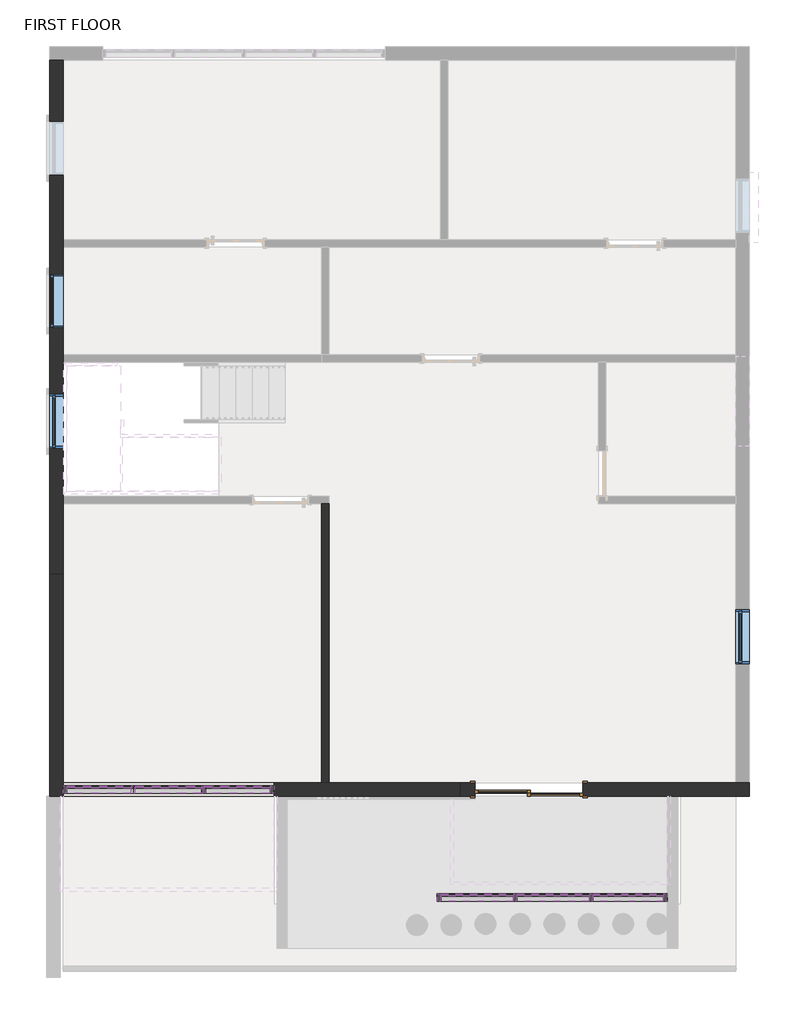
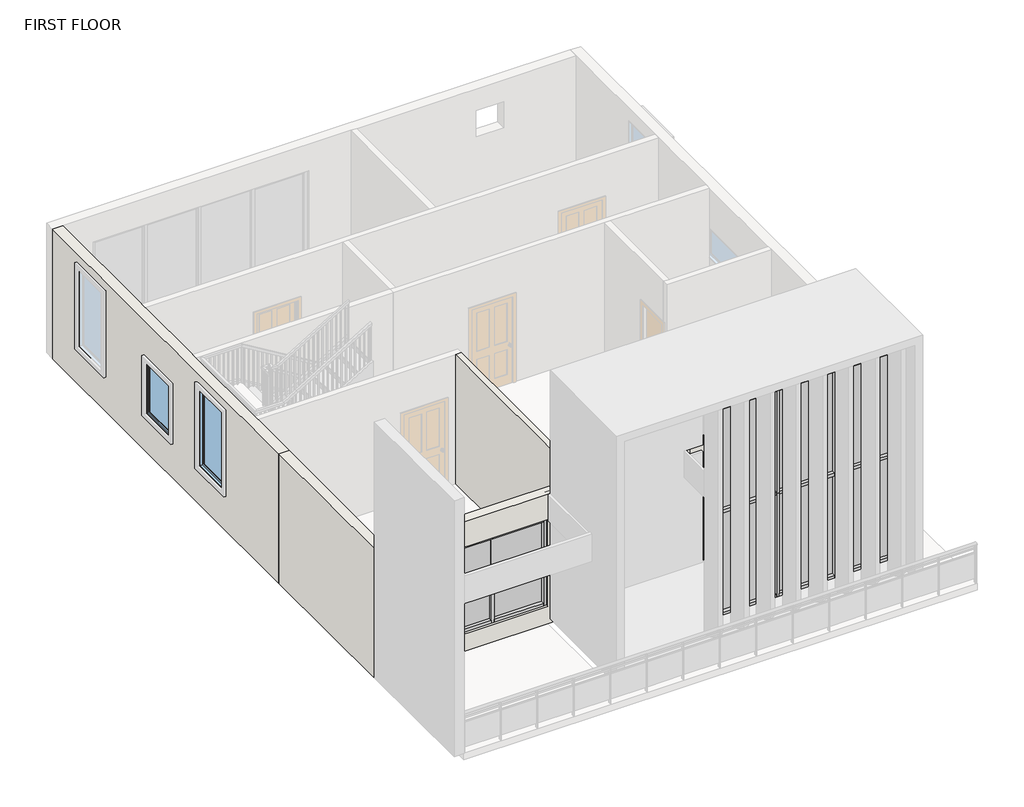
# One storey, part 1 of 4: 42 members, 15 plates, 6 walls, 3 windows, 1 door.
"""IFC4 building model written with IfcOpenShell, lengths in millimetres."""

from ifc_helpers import new_model, si_unit, frame, origin, place, context, project, spatial, polyline, outline, extrude, faceted_brep, transform, mapped, element, save
from components import door_d4d75d1e, member_f0fea5a5, member_ee409385, member_9476229c, member_234fa6b3, member_c6549b41, member_65ceef43, member_37269937, member_65519335, member_c344cd1a, member_3285b992, member_9e1336f4, member_2c52e315, member_a24dc69d, member_2a256751, member_8c482a5e, member_f4ce465c, member_cd6cc0cf, system_panel_glazed_74eece19, system_panel_glazed_8fc2b39e, system_panel_glazed_e38def25, system_panel_glazed_5eb7606f, system_panel_glazed_a48af828, system_panel_glazed_d044bda1, system_panel_glazed_a4577834, system_panel_glazed_3aabc813, system_panel_glazed_a3f6c58c, system_panel_glazed_533eadb3, system_panel_glazed_eb972c8e, system_panel_glazed_22820276, window_c1f32544, window_2e8ca8a3

model = new_model("IFC4")

# Units and contexts
model_context = context("Model", 3, world=origin())
ifc_project = project(units=[si_unit("LENGTHUNIT", "METRE", prefix="MILLI")], contexts=[model_context])

# Site, building, storey
site = spatial("IfcSite", under=ifc_project)
building = spatial("IfcBuilding", under=site)
storey = spatial("IfcBuildingStorey", under=building, Name="FIRST FLOOR", Elevation=3352.8)

# Door
placement = place(None, origin())
door_shape = door_d4d75d1e(model_context)
element("IfcDoor", 1, ObjectType="Door-Double-Sliding : 72\" x 84\"", at=placement, inside=storey, context=model_context, shape_type="MappedRepresentation", body=[
    mapped(door_shape, transform((-1851.8781265, -4147.9142532, 3352.8), x_axis=(-1.0, 0.0, 0.0), y_axis=(0.0, -1.0, 0.0), z_axis=(0.0, 0.0, 1.0))),
])

# Members
member_shape = member_f0fea5a5(model_context)
element("IfcMember", 2, ObjectType="Rectangular Mullion : 2.5\" x 5\" rectangular", at=placement, inside=storey, context=model_context, shape_type="MappedRepresentation", body=[
    mapped(member_shape, transform((-3373.3381264, -6103.7142532, 3631.9550828), x_axis=(1.0, 0.0, 0.0), y_axis=(0.0, -1.0, 0.0), z_axis=(0.0, 0.0, -1.0))),
])
element("IfcMember", 3, ObjectType="Rectangular Mullion : 2.5\" x 5\" rectangular", at=placement, inside=storey, context=model_context, shape_type="MappedRepresentation", body=[
    mapped(member_shape, transform((-2083.0181265, -6103.7142532, 3631.9550828), x_axis=(1.0, 0.0, 0.0), y_axis=(0.0, -1.0, 0.0), z_axis=(0.0, 0.0, -1.0))),
])
element("IfcMember", 4, ObjectType="Rectangular Mullion : 2.5\" x 5\" rectangular", at=placement, inside=storey, context=model_context, shape_type="MappedRepresentation", body=[
    mapped(member_shape, transform((-792.6981266, -6103.7142532, 3631.9550828), x_axis=(1.0, 0.0, 0.0), y_axis=(0.0, -1.0, 0.0), z_axis=(0.0, 0.0, -1.0))),
])
element("IfcMember", 5, ObjectType="Rectangular Mullion : 2.5\" x 5\" rectangular", at=placement, inside=storey, context=model_context, shape_type="MappedRepresentation", body=[
    mapped(member_shape, transform((-3373.3381264, -6103.7142532, 6070.3550828), x_axis=(1.0, 0.0, 0.0), y_axis=(0.0, -1.0, 0.0), z_axis=(0.0, 0.0, -1.0))),
])
element("IfcMember", 6, ObjectType="Rectangular Mullion : 2.5\" x 5\" rectangular", at=placement, inside=storey, context=model_context, shape_type="MappedRepresentation", body=[
    mapped(member_shape, transform((-2083.0181265, -6103.7142532, 6070.3550828), x_axis=(1.0, 0.0, 0.0), y_axis=(0.0, -1.0, 0.0), z_axis=(0.0, 0.0, -1.0))),
])
element("IfcMember", 7, ObjectType="Rectangular Mullion : 2.5\" x 5\" rectangular", at=placement, inside=storey, context=model_context, shape_type="MappedRepresentation", body=[
    mapped(member_shape, transform((-792.6981266, -6103.7142532, 6070.3550828), x_axis=(1.0, 0.0, 0.0), y_axis=(0.0, -1.0, 0.0), z_axis=(0.0, 0.0, -1.0))),
])
member_2_shape = member_ee409385(model_context)
element("IfcMember", 8, ObjectType="Rectangular Mullion : 2.5\" x 5\" rectangular", at=placement, inside=storey, context=model_context, shape_type="MappedRepresentation", body=[
    mapped(member_2_shape, transform((497.6218735, -6103.7142532, 3631.9550828), x_axis=(1.0, 0.0, 0.0), y_axis=(0.0, -1.0, 0.0), z_axis=(0.0, 0.0, -1.0))),
])
element("IfcMember", 9, ObjectType="Rectangular Mullion : 2.5\" x 5\" rectangular", at=placement, inside=storey, context=model_context, shape_type="MappedRepresentation", body=[
    mapped(member_2_shape, transform((497.6218735, -6103.7142532, 6070.3550828), x_axis=(1.0, 0.0, 0.0), y_axis=(0.0, -1.0, 0.0), z_axis=(0.0, 0.0, -1.0))),
])
element("IfcMember", 10, ObjectType="Rectangular Mullion : 2.5\" x 5\" rectangular", at=placement, inside=storey, context=model_context, shape_type="MappedRepresentation", body=[
    mapped(member_2_shape, transform((-3413.9781265, -6103.7142532, 6070.3550828), x_axis=(-1.0, 0.0, 0.0), y_axis=(0.0, -1.0, 0.0), z_axis=(0.0, 0.0, 1.0))),
])
element("IfcMember", 11, ObjectType="Rectangular Mullion : 2.5\" x 5\" rectangular", at=placement, inside=storey, context=model_context, shape_type="MappedRepresentation", body=[
    mapped(member_2_shape, transform((-3413.9781265, -6103.7142532, 8508.7550828), x_axis=(-1.0, 0.0, 0.0), y_axis=(0.0, -1.0, 0.0), z_axis=(0.0, 0.0, 1.0))),
])
member_3_shape = member_9476229c(model_context)
element("IfcMember", 12, ObjectType="Rectangular Mullion : 2.5\" x 5\" rectangular", at=placement, inside=storey, context=model_context, shape_type="MappedRepresentation", body=[
    mapped(member_3_shape, transform((434.1218735, -6103.7142532, 9132.458551), x_axis=(0.0, 0.0, 1.0), y_axis=(0.0, -1.0, 0.0), z_axis=(1.0, 0.0, 0.0))),
])
element("IfcMember", 13, ObjectType="Rectangular Mullion : 2.5\" x 5\" rectangular", at=placement, inside=storey, context=model_context, shape_type="MappedRepresentation", body=[
    mapped(member_3_shape, transform((-760.9481266, -6103.7142532, 3631.9550828), x_axis=(0.0, 0.0, -1.0), y_axis=(0.0, -1.0, 0.0), z_axis=(-1.0, 0.0, 0.0))),
])
member_4_shape = member_234fa6b3(model_context)
element("IfcMember", 14, ObjectType="Rectangular Mullion : 2.5\" x 5\" rectangular", at=placement, inside=storey, context=model_context, shape_type="MappedRepresentation", body=[
    mapped(member_4_shape, transform((-2114.7681265, -6103.7142532, 9132.458551), x_axis=(0.0, 0.0, 1.0), y_axis=(0.0, -1.0, 0.0), z_axis=(1.0, 0.0, 0.0))),
])
element("IfcMember", 15, ObjectType="Rectangular Mullion : 2.5\" x 5\" rectangular", at=placement, inside=storey, context=model_context, shape_type="MappedRepresentation", body=[
    mapped(member_4_shape, transform((-824.4481266, -6103.7142532, 9132.458551), x_axis=(0.0, 0.0, 1.0), y_axis=(0.0, -1.0, 0.0), z_axis=(1.0, 0.0, 0.0))),
])
element("IfcMember", 16, ObjectType="Rectangular Mullion : 2.5\" x 5\" rectangular", at=placement, inside=storey, context=model_context, shape_type="MappedRepresentation", body=[
    mapped(member_4_shape, transform((-3341.5881264, -6103.7142532, 3631.9550828), x_axis=(0.0, 0.0, -1.0), y_axis=(0.0, -1.0, 0.0), z_axis=(-1.0, 0.0, 0.0))),
])
element("IfcMember", 17, ObjectType="Rectangular Mullion : 2.5\" x 5\" rectangular", at=placement, inside=storey, context=model_context, shape_type="MappedRepresentation", body=[
    mapped(member_4_shape, transform((-2051.2681265, -6103.7142532, 3631.9550828), x_axis=(0.0, 0.0, -1.0), y_axis=(0.0, -1.0, 0.0), z_axis=(-1.0, 0.0, 0.0))),
])
member_5_shape = member_c6549b41(model_context)
element("IfcMember", 18, ObjectType="Rectangular Mullion : 2.5\" x 5\" rectangular", at=placement, inside=storey, context=model_context, shape_type="MappedRepresentation", body=[
    mapped(member_5_shape, transform((434.1218735, -6103.7142532, 6070.3550828), x_axis=(0.0, 0.0, 1.0), y_axis=(0.0, -1.0, 0.0), z_axis=(1.0, 0.0, 0.0))),
])
element("IfcMember", 19, ObjectType="Rectangular Mullion : 2.5\" x 5\" rectangular", at=placement, inside=storey, context=model_context, shape_type="MappedRepresentation", body=[
    mapped(member_5_shape, transform((434.1218735, -6103.7142532, 8508.7550828), x_axis=(0.0, 0.0, 1.0), y_axis=(0.0, -1.0, 0.0), z_axis=(1.0, 0.0, 0.0))),
])
member_6_shape = member_65ceef43(model_context)
element("IfcMember", 20, ObjectType="Rectangular Mullion : 2.5\" x 5\" rectangular", at=placement, inside=storey, context=model_context, shape_type="MappedRepresentation", body=[
    mapped(member_6_shape, transform((-2114.7681265, -6103.7142532, 6070.3550828), x_axis=(0.0, 0.0, 1.0), y_axis=(0.0, -1.0, 0.0), z_axis=(1.0, 0.0, 0.0))),
])
element("IfcMember", 21, ObjectType="Rectangular Mullion : 2.5\" x 5\" rectangular", at=placement, inside=storey, context=model_context, shape_type="MappedRepresentation", body=[
    mapped(member_6_shape, transform((-824.4481266, -6103.7142532, 6070.3550828), x_axis=(0.0, 0.0, 1.0), y_axis=(0.0, -1.0, 0.0), z_axis=(1.0, 0.0, 0.0))),
])
element("IfcMember", 22, ObjectType="Rectangular Mullion : 2.5\" x 5\" rectangular", at=placement, inside=storey, context=model_context, shape_type="MappedRepresentation", body=[
    mapped(member_6_shape, transform((-2114.7681265, -6103.7142532, 8508.7550828), x_axis=(0.0, 0.0, 1.0), y_axis=(0.0, -1.0, 0.0), z_axis=(1.0, 0.0, 0.0))),
])
element("IfcMember", 23, ObjectType="Rectangular Mullion : 2.5\" x 5\" rectangular", at=placement, inside=storey, context=model_context, shape_type="MappedRepresentation", body=[
    mapped(member_6_shape, transform((-824.4481266, -6103.7142532, 8508.7550828), x_axis=(0.0, 0.0, 1.0), y_axis=(0.0, -1.0, 0.0), z_axis=(1.0, 0.0, 0.0))),
])
member_7_shape = member_37269937(model_context)
element("IfcMember", 24, ObjectType="Rectangular Mullion : 2.5\" x 5\" rectangular", at=placement, inside=storey, context=model_context, shape_type="MappedRepresentation", body=[
    mapped(member_7_shape, transform((-8601.9281264, -4274.9142532, 5803.9276882), x_axis=(0.0, 0.0, 1.0), y_axis=(0.0, -1.0, 0.0), z_axis=(1.0, 0.0, 0.0))),
])
element("IfcMember", 25, ObjectType="Rectangular Mullion : 2.5\" x 5\" rectangular", at=placement, inside=storey, context=model_context, shape_type="MappedRepresentation", body=[
    mapped(member_7_shape, transform((-7344.6281266, -4274.9142532, 3762.7354604), x_axis=(0.0, 0.0, -1.0), y_axis=(0.0, -1.0, 0.0), z_axis=(-1.0, 0.0, 0.0))),
])
member_8_shape = member_65519335(model_context)
element("IfcMember", 26, ObjectType="Rectangular Mullion : 2.5\" x 5\" rectangular", at=placement, inside=storey, context=model_context, shape_type="MappedRepresentation", body=[
    mapped(member_8_shape, transform((-8601.9281264, -4274.9142532, 4678.4352429), x_axis=(0.0, 0.0, 1.0), y_axis=(0.0, -1.0, 0.0), z_axis=(1.0, 0.0, 0.0))),
])
element("IfcMember", 27, ObjectType="Rectangular Mullion : 2.5\" x 5\" rectangular", at=placement, inside=storey, context=model_context, shape_type="MappedRepresentation", body=[
    mapped(member_8_shape, transform((-6246.0781265, -4274.9142532, 4678.4352429), x_axis=(0.0, 0.0, 1.0), y_axis=(0.0, -1.0, 0.0), z_axis=(1.0, 0.0, 0.0))),
])
member_9_shape = member_c344cd1a(model_context)
element("IfcMember", 28, ObjectType="Rectangular Mullion : 2.5\" x 5\" rectangular", at=placement, inside=storey, context=model_context, shape_type="MappedRepresentation", body=[
    mapped(member_9_shape, transform((-7408.1281266, -4274.9142532, 4678.4352429), x_axis=(0.0, 0.0, 1.0), y_axis=(0.0, -1.0, 0.0), z_axis=(1.0, 0.0, 0.0))),
])
member_10_shape = member_3285b992(model_context)
element("IfcMember", 29, ObjectType="Rectangular Mullion : 2.5\" x 5\" rectangular", at=placement, inside=storey, context=model_context, shape_type="MappedRepresentation", body=[
    mapped(member_10_shape, transform((-9700.4781265, -4274.9142532, 3762.7354604), x_axis=(0.0, 0.0, -1.0), y_axis=(0.0, -1.0, 0.0), z_axis=(-1.0, 0.0, 0.0))),
])
member_11_shape = member_9e1336f4(model_context)
element("IfcMember", 30, ObjectType="Rectangular Mullion : 2.5\" x 5\" rectangular", at=placement, inside=storey, context=model_context, shape_type="MappedRepresentation", body=[
    mapped(member_11_shape, transform((-8570.1781264, -4274.9142532, 3762.7354604), x_axis=(0.0, 0.0, -1.0), y_axis=(0.0, -1.0, 0.0), z_axis=(-1.0, 0.0, 0.0))),
])
element("IfcMember", 31, ObjectType="Rectangular Mullion : 2.5\" x 5\" rectangular", at=placement, inside=storey, context=model_context, shape_type="MappedRepresentation", body=[
    mapped(member_10_shape, transform((-6246.0781265, -4274.9142532, 5803.9276882), x_axis=(0.0, 0.0, 1.0), y_axis=(0.0, -1.0, 0.0), z_axis=(1.0, 0.0, 0.0))),
])
element("IfcMember", 32, ObjectType="Rectangular Mullion : 2.5\" x 5\" rectangular", at=placement, inside=storey, context=model_context, shape_type="MappedRepresentation", body=[
    mapped(member_11_shape, transform((-7376.3781266, -4274.9142532, 5803.9276882), x_axis=(0.0, 0.0, 1.0), y_axis=(0.0, -1.0, 0.0), z_axis=(1.0, 0.0, 0.0))),
])
member_12_shape = member_2c52e315(model_context)
element("IfcMember", 33, ObjectType="Rectangular Mullion : 2.5\" x 5\" rectangular", at=placement, inside=storey, context=model_context, shape_type="MappedRepresentation", body=[
    mapped(member_12_shape, transform((-6182.5781265, -4274.9142532, 3762.7354604), x_axis=(1.0, 0.0, 0.0), y_axis=(0.0, -1.0, 0.0), z_axis=(0.0, 0.0, -1.0))),
])
element("IfcMember", 34, ObjectType="Rectangular Mullion : 2.5\" x 5\" rectangular", at=placement, inside=storey, context=model_context, shape_type="MappedRepresentation", body=[
    mapped(member_12_shape, transform((-9763.9781265, -4274.9142532, 4678.4352429), x_axis=(-1.0, 0.0, 0.0), y_axis=(0.0, -1.0, 0.0), z_axis=(0.0, 0.0, 1.0))),
])
member_13_shape = member_a24dc69d(model_context)
element("IfcMember", 35, ObjectType="Rectangular Mullion : 2.5\" x 5\" rectangular", at=placement, inside=storey, context=model_context, shape_type="MappedRepresentation", body=[
    mapped(member_13_shape, transform((-7376.3781266, -4274.9142532, 3762.7354604), x_axis=(1.0, 0.0, 0.0), y_axis=(0.0, -1.0, 0.0), z_axis=(0.0, 0.0, -1.0))),
])
member_14_shape = member_2a256751(model_context)
element("IfcMember", 36, ObjectType="Rectangular Mullion : 2.5\" x 5\" rectangular", at=placement, inside=storey, context=model_context, shape_type="MappedRepresentation", body=[
    mapped(member_14_shape, transform((-3373.3381264, -6103.7142532, 8508.7550828), x_axis=(1.0, 0.0, 0.0), y_axis=(0.0, -1.0, 0.0), z_axis=(0.0, 0.0, -1.0))),
])
element("IfcMember", 37, ObjectType="Rectangular Mullion : 2.5\" x 5\" rectangular", at=placement, inside=storey, context=model_context, shape_type="MappedRepresentation", body=[
    mapped(member_14_shape, transform((-2083.0181265, -6103.7142532, 8508.7550828), x_axis=(1.0, 0.0, 0.0), y_axis=(0.0, -1.0, 0.0), z_axis=(0.0, 0.0, -1.0))),
])
element("IfcMember", 38, ObjectType="Rectangular Mullion : 2.5\" x 5\" rectangular", at=placement, inside=storey, context=model_context, shape_type="MappedRepresentation", body=[
    mapped(member_14_shape, transform((-792.6981266, -6103.7142532, 8508.7550828), x_axis=(1.0, 0.0, 0.0), y_axis=(0.0, -1.0, 0.0), z_axis=(0.0, 0.0, -1.0))),
])
member_15_shape = member_8c482a5e(model_context)
element("IfcMember", 39, ObjectType="Rectangular Mullion : 2.5\" x 5\" rectangular", at=placement, inside=storey, context=model_context, shape_type="MappedRepresentation", body=[
    mapped(member_15_shape, transform((-3413.9781265, -6103.7142532, 9132.458551), x_axis=(-1.0, 0.0, 0.0), y_axis=(0.0, -1.0, 0.0), z_axis=(0.0, 0.0, 1.0))),
])
element("IfcMember", 40, ObjectType="Rectangular Mullion : 2.5\" x 5\" rectangular", at=placement, inside=storey, context=model_context, shape_type="MappedRepresentation", body=[
    mapped(member_15_shape, transform((497.6218735, -6103.7142532, 8508.7550828), x_axis=(1.0, 0.0, 0.0), y_axis=(0.0, -1.0, 0.0), z_axis=(0.0, 0.0, -1.0))),
])
member_16_shape = member_f4ce465c(model_context)
element("IfcMember", 41, ObjectType="Rectangular Mullion : 2.5\" x 5\" rectangular", at=placement, inside=storey, context=model_context, shape_type="MappedRepresentation", body=[
    mapped(member_16_shape, transform((-8570.1781264, -4274.9142532, 4646.6852429), x_axis=(1.0, 0.0, 0.0), y_axis=(0.0, -1.0, 0.0), z_axis=(0.0, 0.0, -1.0))),
])
member_17_shape = member_cd6cc0cf(model_context)
element("IfcMember", 42, ObjectType="Rectangular Mullion : 2.5\" x 5\" rectangular", at=placement, inside=storey, context=model_context, shape_type="MappedRepresentation", body=[
    mapped(member_17_shape, transform((-9763.9781265, -4274.9142532, 5803.9276882), x_axis=(-1.0, 0.0, 0.0), y_axis=(0.0, -1.0, 0.0), z_axis=(0.0, 0.0, 1.0))),
])
element("IfcMember", 43, ObjectType="Rectangular Mullion : 2.5\" x 5\" rectangular", at=placement, inside=storey, context=model_context, shape_type="MappedRepresentation", body=[
    mapped(member_17_shape, transform((-6182.5781265, -4274.9142532, 4678.4352429), x_axis=(1.0, 0.0, 0.0), y_axis=(0.0, -1.0, 0.0), z_axis=(0.0, 0.0, -1.0))),
])

# Plates
system_panel_glazed_shape = system_panel_glazed_74eece19(model_context)
element("IfcPlate", 44, ObjectType="System Panel : Glazed", at=placement, inside=storey, context=model_context, shape_type="MappedRepresentation", body=[
    mapped(system_panel_glazed_shape, transform((-163.4131266, -6103.7142532, 3695.4550828), x_axis=(1.0, 0.0, 0.0), y_axis=(0.0, 1.0, 0.0), z_axis=(0.0, 0.0, 1.0))),
])
system_panel_glazed_2_shape = system_panel_glazed_8fc2b39e(model_context)
element("IfcPlate", 45, ObjectType="System Panel : Glazed", at=placement, inside=storey, context=model_context, shape_type="MappedRepresentation", body=[
    mapped(system_panel_glazed_2_shape, transform((-2728.1781265, -6103.7142532, 3695.4550828), x_axis=(1.0, 0.0, 0.0), y_axis=(0.0, 1.0, 0.0), z_axis=(0.0, 0.0, 1.0))),
])
element("IfcPlate", 46, ObjectType="System Panel : Glazed", at=placement, inside=storey, context=model_context, shape_type="MappedRepresentation", body=[
    mapped(system_panel_glazed_2_shape, transform((-1437.8581266, -6103.7142532, 3695.4550828), x_axis=(1.0, 0.0, 0.0), y_axis=(0.0, 1.0, 0.0), z_axis=(0.0, 0.0, 1.0))),
])
system_panel_glazed_3_shape = system_panel_glazed_e38def25(model_context)
element("IfcPlate", 47, ObjectType="System Panel : Glazed", at=placement, inside=storey, context=model_context, shape_type="MappedRepresentation", body=[
    mapped(system_panel_glazed_3_shape, transform((-163.4131266, -6103.7142532, 6102.1050828), x_axis=(1.0, 0.0, 0.0), y_axis=(0.0, 1.0, 0.0), z_axis=(0.0, 0.0, 1.0))),
])
system_panel_glazed_4_shape = system_panel_glazed_5eb7606f(model_context)
element("IfcPlate", 48, ObjectType="System Panel : Glazed", at=placement, inside=storey, context=model_context, shape_type="MappedRepresentation", body=[
    mapped(system_panel_glazed_4_shape, transform((-2728.1781265, -6103.7142532, 6102.1050828), x_axis=(1.0, 0.0, 0.0), y_axis=(0.0, 1.0, 0.0), z_axis=(0.0, 0.0, 1.0))),
])
element("IfcPlate", 49, ObjectType="System Panel : Glazed", at=placement, inside=storey, context=model_context, shape_type="MappedRepresentation", body=[
    mapped(system_panel_glazed_4_shape, transform((-1437.8581266, -6103.7142532, 6102.1050828), x_axis=(1.0, 0.0, 0.0), y_axis=(0.0, 1.0, 0.0), z_axis=(0.0, 0.0, 1.0))),
])
system_panel_glazed_5_shape = system_panel_glazed_a48af828(model_context)
element("IfcPlate", 50, ObjectType="System Panel : Glazed", at=placement, inside=storey, context=model_context, shape_type="MappedRepresentation", body=[
    mapped(system_panel_glazed_5_shape, transform((-6795.3531265, -4274.9142532, 3826.2354604), x_axis=(1.0, 0.0, 0.0), y_axis=(0.0, 1.0, 0.0), z_axis=(0.0, 0.0, 1.0))),
])
system_panel_glazed_6_shape = system_panel_glazed_d044bda1(model_context)
element("IfcPlate", 51, ObjectType="System Panel : Glazed", at=placement, inside=storey, context=model_context, shape_type="MappedRepresentation", body=[
    mapped(system_panel_glazed_6_shape, transform((-9135.3281264, -4274.9142532, 3826.2354604), x_axis=(1.0, 0.0, 0.0), y_axis=(0.0, 1.0, 0.0), z_axis=(0.0, 0.0, 1.0))),
])
system_panel_glazed_7_shape = system_panel_glazed_a4577834(model_context)
element("IfcPlate", 52, ObjectType="System Panel : Glazed", at=placement, inside=storey, context=model_context, shape_type="MappedRepresentation", body=[
    mapped(system_panel_glazed_7_shape, transform((-7989.1531265, -4274.9142532, 3826.2354604), x_axis=(1.0, 0.0, 0.0), y_axis=(0.0, 1.0, 0.0), z_axis=(0.0, 0.0, 1.0))),
])
system_panel_glazed_8_shape = system_panel_glazed_3aabc813(model_context)
element("IfcPlate", 53, ObjectType="System Panel : Glazed", at=placement, inside=storey, context=model_context, shape_type="MappedRepresentation", body=[
    mapped(system_panel_glazed_8_shape, transform((-163.4131266, -6103.7142532, 8540.5050828), x_axis=(1.0, 0.0, 0.0), y_axis=(0.0, 1.0, 0.0), z_axis=(0.0, 0.0, 1.0))),
])
system_panel_glazed_9_shape = system_panel_glazed_a3f6c58c(model_context)
element("IfcPlate", 54, ObjectType="System Panel : Glazed", at=placement, inside=storey, context=model_context, shape_type="MappedRepresentation", body=[
    mapped(system_panel_glazed_9_shape, transform((-2728.1781265, -6103.7142532, 8540.5050828), x_axis=(1.0, 0.0, 0.0), y_axis=(0.0, 1.0, 0.0), z_axis=(0.0, 0.0, 1.0))),
])
element("IfcPlate", 55, ObjectType="System Panel : Glazed", at=placement, inside=storey, context=model_context, shape_type="MappedRepresentation", body=[
    mapped(system_panel_glazed_9_shape, transform((-1437.8581266, -6103.7142532, 8540.5050828), x_axis=(1.0, 0.0, 0.0), y_axis=(0.0, 1.0, 0.0), z_axis=(0.0, 0.0, 1.0))),
])
system_panel_glazed_10_shape = system_panel_glazed_533eadb3(model_context)
element("IfcPlate", 56, ObjectType="System Panel : Glazed", at=placement, inside=storey, context=model_context, shape_type="MappedRepresentation", body=[
    mapped(system_panel_glazed_10_shape, transform((-9151.2031264, -4274.9142532, 4710.1852429), x_axis=(1.0, 0.0, 0.0), y_axis=(0.0, 1.0, 0.0), z_axis=(0.0, 0.0, 1.0))),
])
system_panel_glazed_11_shape = system_panel_glazed_eb972c8e(model_context)
element("IfcPlate", 57, ObjectType="System Panel : Glazed", at=placement, inside=storey, context=model_context, shape_type="MappedRepresentation", body=[
    mapped(system_panel_glazed_11_shape, transform((-7957.4031265, -4274.9142532, 4710.1852429), x_axis=(1.0, 0.0, 0.0), y_axis=(0.0, 1.0, 0.0), z_axis=(0.0, 0.0, 1.0))),
])
system_panel_glazed_12_shape = system_panel_glazed_22820276(model_context)
element("IfcPlate", 58, ObjectType="System Panel : Glazed", at=placement, inside=storey, context=model_context, shape_type="MappedRepresentation", body=[
    mapped(system_panel_glazed_12_shape, transform((-6811.2281265, -4274.9142532, 4710.1852429), x_axis=(1.0, 0.0, 0.0), y_axis=(0.0, 1.0, 0.0), z_axis=(0.0, 0.0, 1.0))),
])

# Walls
element("IfcWall", 59, ObjectType="INNER WALL THICKNESS 5\"", at=placement, inside=storey, context=model_context, shape_type="SweptSolid", body=[
    extrude(outline(polyline([(-5369.7781265, -4160.6142532), (-5369.7781265, 576.1165128), (-5242.7781265, 576.1165128), (-5242.7781265, -4160.6142532), (-5369.7781265, -4160.6142532)])), frame((0.0, 0.0, 3352.8), z_axis=(0.0, 0.0, 1.0), x_axis=(1.0, 0.0, 0.0)), (0.0, 0.0, 1.0), 3048.0),
])
element("IfcWall", 60, ObjectType="OUTER WALL THICKNESS 9\"", at=placement, inside=storey, context=model_context, shape_type="Brep", body=[
    faceted_brep([(-3020.2781265, -4389.2142532, 3352.8), (-2766.2781265, -4389.2142532, 3352.8), (-2766.2781265, -4389.2142532, 5486.4), (-937.4781265, -4389.2142532, 5486.4), (-937.4781265, -4389.2142532, 3352.8), (1894.6218735, -4389.2142532, 3352.8), (1894.6218735, -4389.2142532, 6400.8), (-3020.2781265, -4389.2142532, 6400.8), (-2766.2781265, -4160.6142532, 5486.4), (-2766.2781265, -4160.6142532, 3352.8), (-3020.2781265, -4160.6142532, 3352.8), (-3020.2781265, -4160.6142532, 6400.8), (1666.0218735, -4160.6142532, 6400.8), (1894.6218735, -4160.6142532, 6400.8), (1894.6218735, -4160.6142532, 3352.8), (1666.0218735, -4160.6142532, 3352.8), (-937.4781265, -4160.6142532, 3352.8), (-937.4781265, -4160.6142532, 5486.4)], [[[0, 1, 2, 3, 4, 5, 6, 7]], [[8, 9, 10, 11, 12, 13, 14, 15, 16, 17]], [[10, 9, 1, 0]], [[16, 15, 14, 5, 4]], [[7, 6, 13, 12, 11]], [[0, 7, 11, 10]], [[4, 3, 17, 16]], [[2, 1, 9, 8]], [[3, 2, 8, 17]], [[6, 5, 14, 13]]]),
])
element("IfcWall", 61, ObjectType="OUTER WALL THICKNESS 9\"", at=placement, inside=storey, context=model_context, shape_type="Brep", body=[
    faceted_brep([(-9992.5781265, 8107.5857468, 3352.8), (-9992.5781265, -617.3142532, 3352.8), (-9992.5781265, -617.3142532, 6400.8), (-9992.5781265, 8107.5857468, 6400.8), (-9992.5781265, 7066.1857468, 6096.0), (-9992.5781265, 6151.7857468, 6096.0), (-9992.5781265, 6151.7857468, 4267.2), (-9992.5781265, 7066.1857468, 4267.2), (-9992.5781265, 2430.6857468, 6096.0), (-9992.5781265, 1516.2857468, 6096.0), (-9992.5781265, 1516.2857468, 4267.2), (-9992.5781265, 2430.6857468, 4267.2), (-9992.5781265, 4475.3857468, 5486.4), (-9992.5781265, 3560.9857468, 5486.4), (-9992.5781265, 3560.9857468, 4267.2), (-9992.5781265, 4475.3857468, 4267.2), (-9763.9781265, 8107.5857468, 3352.8), (-9763.9781265, 8107.5857468, 6400.8), (-9763.9781265, 5059.5857468, 6400.8), (-9763.9781265, 4932.5857468, 6400.8), (-9763.9781265, 3103.7857468, 6400.8), (-9763.9781265, 2976.7857468, 6400.8), (-9763.9781265, 703.1165128, 6400.8), (-9763.9781265, 576.1165128, 6400.8), (-9763.9781265, -617.3142532, 6400.8), (-9763.9781265, -617.3142532, 3352.8), (-9763.9781265, 576.1165128, 3352.8), (-9763.9781265, 703.1165128, 3352.8), (-9763.9781265, 2976.7857468, 3352.8), (-9763.9781265, 3103.7857468, 3352.8), (-9763.9781265, 4932.5857468, 3352.8), (-9763.9781265, 5059.5857468, 3352.8), (-9763.9781265, 7066.1857468, 6096.0), (-9763.9781265, 7066.1857468, 4267.2), (-9763.9781265, 6151.7857468, 4267.2), (-9763.9781265, 6151.7857468, 6096.0), (-9763.9781265, 2430.6857468, 6096.0), (-9763.9781265, 2430.6857468, 4267.2), (-9763.9781265, 1516.2857468, 4267.2), (-9763.9781265, 1516.2857468, 6096.0), (-9763.9781265, 4475.3857468, 5486.4), (-9763.9781265, 4475.3857468, 4267.2), (-9763.9781265, 3560.9857468, 4267.2), (-9763.9781265, 3560.9857468, 5486.4)], [[[0, 1, 2, 3], [4, 5, 6, 7], [8, 9, 10, 11], [12, 13, 14, 15]], [[16, 17, 18, 19, 20, 21, 22, 23, 24, 25, 26, 27, 28, 29, 30, 31], [32, 33, 34, 35], [36, 37, 38, 39], [40, 41, 42, 43]], [[1, 0, 16, 31, 30, 29, 28, 27, 26, 25]], [[2, 1, 25, 24]], [[3, 2, 24, 23, 22, 21, 20, 19, 18, 17]], [[0, 3, 17, 16]], [[33, 32, 4, 7]], [[34, 33, 7, 6]], [[35, 34, 6, 5]], [[32, 35, 5, 4]], [[37, 36, 8, 11]], [[38, 37, 11, 10]], [[39, 38, 10, 9]], [[36, 39, 9, 8]], [[41, 40, 12, 15]], [[42, 41, 15, 14]], [[43, 42, 14, 13]], [[40, 43, 13, 12]]]),
])
element("IfcWall", 62, ObjectType="OUTER WALL THICKNESS 9\"", at=placement, inside=storey, context=model_context, shape_type="Brep", body=[
    faceted_brep([(-9992.5781265, -617.3142532, 3352.8), (-9992.5781265, -4389.2142532, 3352.8), (-9992.5781265, -4389.2142532, 6400.8), (-9992.5781265, -617.3142532, 6400.8), (-9763.9781265, -617.3142532, 3352.8), (-9763.9781265, -617.3142532, 6400.8), (-9763.9781265, -4160.6142532, 6400.8), (-9763.9781265, -4389.2142532, 6400.8), (-9763.9781265, -4389.2142532, 6099.8993475), (-9763.9781265, -4389.2142532, 3352.8)], [[[0, 1, 2, 3]], [[4, 5, 6, 7, 8, 9]], [[1, 0, 4, 9]], [[3, 2, 7, 6, 5]], [[0, 3, 5, 4]], [[2, 1, 9, 8, 7]]]),
])
element("IfcWall", 63, ObjectType="OUTER WALL THICKNESS 9\"", at=placement, inside=storey, context=model_context, shape_type="Brep", body=[
    faceted_brep([(-9763.9781265, -4389.2142532, 3352.8), (-3020.2781265, -4389.2142532, 3352.8), (-3020.2781265, -4389.2142532, 6400.8), (-9763.9781265, -4389.2142532, 6400.8), (-9763.9781265, -4389.2142532, 5803.9276882), (-6182.5781265, -4389.2142532, 5803.9276882), (-6182.5781265, -4389.2142532, 3762.7354604), (-9763.9781265, -4389.2142532, 3762.7354604), (-3020.2781265, -4160.6142532, 3352.8), (-5242.7781265, -4160.6142532, 3352.8), (-5369.7781265, -4160.6142532, 3352.8), (-9763.9781265, -4160.6142532, 3352.8), (-9763.9781265, -4160.6142532, 3762.7354604), (-6182.5781265, -4160.6142532, 3762.7354604), (-6182.5781265, -4160.6142532, 5803.9276882), (-9763.9781265, -4160.6142532, 5803.9276882), (-9763.9781265, -4160.6142532, 6400.8), (-5369.7781265, -4160.6142532, 6400.8), (-5242.7781265, -4160.6142532, 6400.8), (-3020.2781265, -4160.6142532, 6400.8)], [[[0, 1, 2, 3, 4, 5, 6, 7]], [[8, 9, 10, 11, 12, 13, 14, 15, 16, 17, 18, 19]], [[1, 0, 11, 10, 9, 8]], [[2, 1, 8, 19]], [[3, 2, 19, 18, 17, 16]], [[3, 16, 15, 4]], [[11, 0, 7, 12]], [[14, 5, 4, 15]], [[5, 14, 13, 6]], [[6, 13, 12, 7]]]),
])
element("IfcWall", 64, ObjectType="OUTER WALL THICKNESS 9\"", at=placement, inside=storey, context=model_context, shape_type="SweptSolid", body=[
    extrude(outline(polyline([(-6182.5781265, -4300.3142532), (-6182.5781265, -4274.9142532), (-5953.9781265, -4274.9142532), (-5953.9781265, -4300.3142532), (-6182.5781265, -4300.3142532)])), frame((0.0, 0.0, 3352.8), z_axis=(0.0, 0.0, 1.0), x_axis=(1.0, 0.0, 0.0)), (0.0, 0.0, 1.0), 3048.0),
])

# Windows
window_shape = window_c1f32544(model_context)
element("IfcWindow", 65, ObjectType="Fixed : 36\" x 48\"", at=placement, inside=storey, context=model_context, shape_type="MappedRepresentation", body=[
    mapped(window_shape, transform((-9878.2781265, 4056.2857468, 3352.8), x_axis=(0.0, 1.0, 0.0), y_axis=(-1.0, 0.0, 0.0), z_axis=(0.0, 0.0, 1.0))),
])
window_2_shape = window_2e8ca8a3(model_context)
element("IfcWindow", 66, ObjectType="Fixed : window 3' x 6\"", at=placement, inside=storey, context=model_context, shape_type="MappedRepresentation", body=[
    mapped(window_2_shape, transform((1780.3218735, -1646.0142532, 3352.8), x_axis=(0.0, 1.0, 0.0), y_axis=(-1.0, 0.0, 0.0), z_axis=(0.0, 0.0, 1.0))),
])
element("IfcWindow", 67, ObjectType="Fixed : window 3' x 6\"", at=placement, inside=storey, context=model_context, shape_type="MappedRepresentation", body=[
    mapped(window_2_shape, transform((-9878.2781265, 2011.5857468, 3352.8), x_axis=(0.0, 1.0, 0.0), y_axis=(-1.0, 0.0, 0.0), z_axis=(0.0, 0.0, 1.0))),
])

save(model, "model.ifc")

# Revit data of these elements
# Type "Door-Double-Sliding : 72\" x 84\""
#   Type Mark = "8"
#   Construction Type Id = "opn-d45"
#   Assembly Code = "C1020"
#   Analytic Construction = "Wood frame, double glass door "
#   Thickness = 0' - 2"
#   Thermal Resistance (R) = 1.8150 (h·ft²·°F)/BTU
#   Heat Transfer Coefficient (U) = 0.5510 BTU/(h·ft²·°F)
#   Height = 7' - 0"
#   Rail Width = 0' - 2"
#   Stiles = 0' - 2"
#   Trim Projection Ext = 0' - 1"
#   Trim Projection Int = 0' - 1"
#   Trim Width = 0' - 3"
#   Width = 6' - 0"
#   Define Thermal Properties by = 1
#   Glazing = Glass
#   Panel Material = Wood - Birch - Solid Stained Light Low Gloss
#   Trim Material = Paint - Sienna
#   Visual Light Transmittance = 0
#   Solar Heat Gain Coefficient = 0
#   Function = (empty or 0)
#   Wall Closure = (empty or 0)
# Type "Rectangular Mullion : 2.5\" x 5\" rectangular"
#   built-in parameter 1007304 = 0.416667 (stored number, unit not read)
#   built-in parameter 1007301 = 0.104167 (stored number, unit not read)
#   built-in parameter 1007300 = 0.104167 (stored number, unit not read)
# Type "System Panel : Glazed"
#   Construction Type Id = "GSP4R"
#   Analytic Construction = "1/8 in Pilkington single glazing"
#   Visual Light Transmittance = 0.9
#   Solar Heat Gain Coefficient = 0.86
#   Heat Transfer Coefficient (U) = 1.18115 BTU/(h·ft²·°F)
#   Define Thermal Properties by = 1
# Type "INNER WALL THICKNESS 5\""
#   Assembly Code = "B2010"
#   Layers, outside or top first: 0' - 5" "WALL PAINT" (function 1)
# Type "OUTER WALL THICKNESS 9\""
#   Assembly Code = "B2010"
#   Layers, outside or top first: 0' - 9" "WALL PAINT" (function 1)
# Type "Fixed : 36\" x 48\""
#   Type Mark = "1"
#   Construction Type Id = "GSP4R"
#   Assembly Code = "B2020100"
#   Analytic Construction = "1/8 in Pilkington single glazing"
#   Visual Light Transmittance = 0.9
#   Solar Heat Gain Coefficient = 0.78
#   Heat Transfer Coefficient (U) = 0.6496 BTU/(h·ft²·°F)
#   Height = 4' - 0"
#   Default Sill Height = 3' - 0"
#   Width = 3' - 0"
#   Window Inset = 0' - 0 3/4"
#   Define Thermal Properties by = 1
#   Define Thermal Properties by = 1
#   Glass Pane Material = Glass
#   Sash Material = Sash
#   Wall Closure = (empty or 0)
# Type "Fixed : window 3' x 6\""
#   Type Mark = "26"
#   Construction Type Id = "GSP4R"
#   Assembly Code = "B2020100"
#   Analytic Construction = "1/8 in Pilkington single glazing"
#   Visual Light Transmittance = 0.9
#   Solar Heat Gain Coefficient = 0.78
#   Heat Transfer Coefficient (U) = 0.6496 BTU/(h·ft²·°F)
#   Height = 6' - 0"
#   Default Sill Height = 3' - 0"
#   Width = 3' - 0"
#   Window Inset = 0' - 2"
#   Define Thermal Properties by = 1
#   Glass Pane Material = Glass
#   Sash Material = Sash
#   Wall Closure = (empty or 0)
# Element 1 (IfcDoor, "Door-Double-Sliding : 72\" x 84\"")
#   Phase Created = New Construction
#   Materials on its faces: "Paint - Sienna", "Wood - Birch - Solid Stained Light Low Gloss", "Glass"
# Elements 2, 3, 4, 5, 6, 7, 8, 9, 10, 11, 12, 13, 14, 15, 16, 17, 18, 19, 20, 21, 22, 23, 24, 25, 26, 27, 28, 29, 30, 31, 32, 33, 34, 35, 36, 37, 38, 39, 40, 41, 42, 43 (IfcMember, "Rectangular Mullion : 2.5\" x 5\" rectangular")
#   Phase Created = New Construction
#   Materials on its faces: "BLACK COLOUR"
# Elements 44, 45, 46, 47, 48, 49, 50, 51, 52, 53, 54, 55, 56, 57, 58 (IfcPlate, "System Panel : Glazed")
#   Phase Created = New Construction
#   Materials on its faces: "Glass"
# Element 59 (IfcWall, "INNER WALL THICKNESS 5\"")
#   Top Offset = 0' - 0"
#   Base Offset = 0' - 0"
#   Unconnected Height = 10' - 0"
#   wall height = 10' - 0"
#   Phase Created = New Construction
#   Base Constraint = FIRST FLOOR
#   Materials on its faces: "WALL PAINT"
# Elements 60, 62, 63, 64 (IfcWall, "OUTER WALL THICKNESS 9\"")
#   Top Offset = 0' - 0"
#   Base Offset = 0' - 0"
#   Unconnected Height = 10' - 0"
#   wall height = 10' - 0"
#   Phase Created = New Construction
#   Base Constraint = FIRST FLOOR
#   Materials on its faces: "WALL PAINT"
# Element 61 (IfcWall, "OUTER WALL THICKNESS 9\"")
#   Top Offset = 0' - 0"
#   Base Offset = 0' - 0"
#   wall height = 10' - 0"
#   Phase Created = New Construction
#   Base Constraint = FIRST FLOOR
#   Top Constraint = SECOND FLR
#   Materials on its faces: "WALL PAINT"
# Element 65 (IfcWindow, "Fixed : 36\" x 48\"")
#   Mark = "25"
#   Phase Created = New Construction
#   Materials on its faces: "Sash", "Glass"
# Element 66 (IfcWindow, "Fixed : window 3' x 6\"")
#   Mark = "8"
#   Phase Created = New Construction
#   Materials on its faces: "Sash", "Glass"
# Element 67 (IfcWindow, "Fixed : window 3' x 6\"")
#   Mark = "23"
#   Phase Created = New Construction
#   Materials on its faces: "Sash", "Glass"
# Materials
#   "Glass": class "Glass", colour RGB 0 128 192, transparency 0.75, Description = "Soda Lime Glass", Cost = 0
#   "Wood - Birch - Solid Stained Light Low Gloss": class "Wood", colour RGB 210 159 95, transparency 0, Cost = 0
#   "Paint - Sienna": colour RGB 118 70 51, transparency 0, Cost = 0
#   "WALL PAINT": class "Generic", colour RGB 120 120 120, transparency 0, Cost = 0
#   "Sash": class "Wood", colour RGB 224 178 126, transparency 0, Cost = 0
#   "BLACK COLOUR": class "Generic", colour RGB 120 120 120, transparency 0, Cost = 0
# Room at (-7592.278, 4018.186) mm, phase "New Construction", upper level "FIRST FLOOR", upper offset 10' - 0", lower offset 0' - 0"
#   Number = "7"
#   Name = "TOILET"
# Room at (-7592.278, -1817.649) mm, phase "New Construction", upper level "FIRST FLOOR", upper offset 10' - 0", lower offset 0' - 0"
#   Number = "8"
#   Name = "BEDROOM"
# Room at (-1762.978, 4018.186) mm, phase "New Construction", upper level "FIRST FLOOR", upper offset 10' - 0", lower offset 0' - 0"
#   Number = "9"
#   Name = "PASSAGE ROOM"
# Room at (-4048.978, -617.314) mm, phase "New Construction", upper level "FIRST FLOOR", upper offset 10' - 0", lower offset 0' - 0"
#   Number = "10"
# Room at (586.522, 1839.951) mm, phase "New Construction", upper level "FIRST FLOOR", upper offset 10' - 0", lower offset 0' - 0"
#   Number = "11"
#   Name = "TOILET"
# Room at (-753.328, 6608.986) mm, phase "New Construction", upper level "FIRST FLOOR", upper offset 10' - 0", lower offset 0' - 0"
#   Number = "12"
# Room at (-6582.628, 6608.986) mm, phase "New Construction", upper level "FIRST FLOOR", upper offset 10' - 0", lower offset 0' - 0"
#   Number = "13"
#   Name = "BEDROOM"
